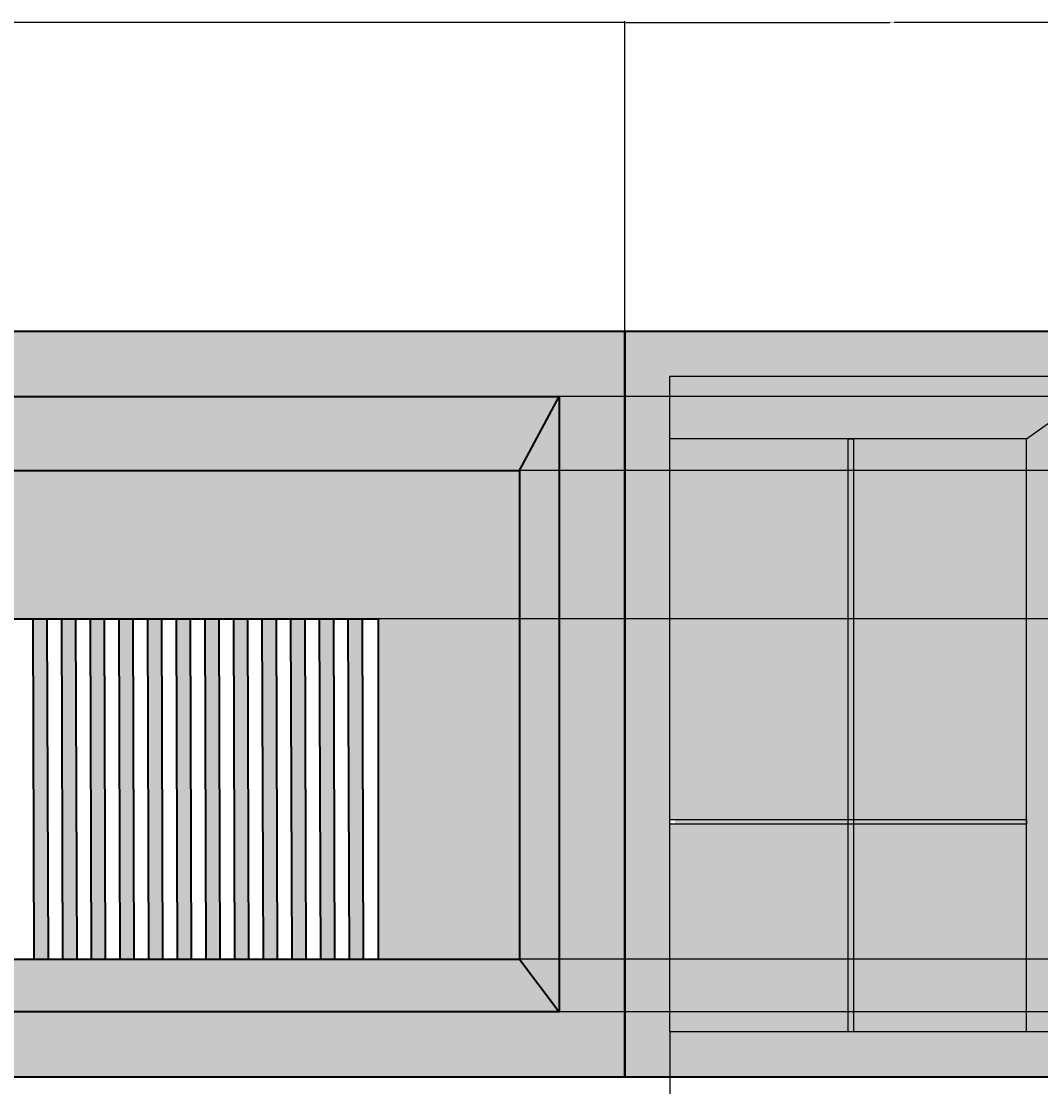
# Model space of a CAD drawing. Units: feet. Extents: x 1141 to 2858, y 751 to 1654.
# Tile 7 of 13: x 1916 to 2096, y 1466 to 1654. Entities that reach past the tile are written whole.
import ezdxf

# ---------------------------------------------------------------- set-up
doc = ezdxf.new("R2010")
doc.units = ezdxf.units.FT
for name, color, linetype, lineweight in [('A-ANNO-DIMS', 2, 'Continuous', 18), ('A-ELEV', 7, 'Continuous', 35), ('A-ELEV-PATT', 8, 'Continuous', 13), ('A-GLAZ', 4, 'Continuous', 25)]:
    doc.layers.add(name, color=color, linetype=linetype, lineweight=lineweight)
doc.styles.get("Standard").update_dxf_attribs({"font": 'arial.ttf'})
doc.dimstyles.get("Standard").update_dxf_attribs({"dimtxt": 0.18, "dimasz": 0.18, "dimexe": 0.18, "dimexo": 0.0625, "dimgap": 0.09, "dimtad": 0, "dimtih": 1, "dimtoh": 1, "dimdec": 1, "dimzin": 0, "dimdsep": 46, "dimlunit": 3, "dimtxsty": 'Standard', "dimcen": 0.09, "dimadec": 0, "dimazin": 0, "dimtfac": 1, "dimtdec": 1, "dimtofl": 0, "dimtmove": 0, "dimatfit": 3, "dimfxl": 1, "dimtolj": 1, "dimtzin": 0, "dimarcsym": 0})

# ---------------------------------------------------------------- blocks, each defined once
blk = doc.blocks.new('WIN-SIDE-A')
blk.add_line((63.09, 104.94), (78.57, 116.03))
blk.add_line((63.09, 104.94), (78.57, 116.03))
for points in [[(78.57, 0), (0, 0), (0, 116.03), (78.57, 116.03)], [(78.57, 0), (0, 0), (0, 116.03), (78.57, 116.03)], [(31.54, 104.94), (32.46, 104.94), (32.46, 0), (31.54, 0)], [(0, 37.61), (63.09, 37.61), (63.09, 36.79), (0, 36.79)]]:
    blk.add_lwpolyline(points, close=True)
for points in [[(63.09, 0), (63.09, 104.94), (0, 104.94)], [(63.09, 0), (63.09, 104.94), (0, 104.94)], [(31.54, 37.61), (31.54, 104.94), (32.46, 104.94), (32.46, 37.61)], [(31.54, 36.79), (0, 36.79), (0, 37.61), (31.54, 37.61)], [(32.46, 36.79), (32.46, 0), (31.54, 0), (31.54, 36.79)], [(32.46, 37.61), (63.09, 37.61), (63.09, 36.79), (32.46, 36.79)]]:
    blk.add_lwpolyline(points)
blk = doc.blocks.new('*D15')
at = {"layer": 'A-ANNO-DIMS', "color": 0, "lineweight": -2, "transparency": 16777216}
for p, q in [((2030.85, 1475.38), (2030.85, 1457.85)), ((2109.42, 1475.38), (2109.42, 1457.85)), ((2031.03, 1458.03), (2069.61, 1458.03)), ((2109.24, 1458.03), (2070.66, 1458.03))]:
    blk.add_line(p, q, dxfattribs=at)
at = {"layer": 'A-ANNO-DIMS', "color": 0, "transparency": 16777216}
for points in [[(2031.03, 1458.06), (2031.03, 1458), (2030.85, 1458.03)], [(2109.24, 1458.06), (2109.24, 1458), (2109.42, 1458.03)]]:
    blk.add_solid(points, dxfattribs=at)
at = {"layer": 'Defpoints', "color": 0, "transparency": 16777216}
for p in [(2030.85, 1475.44), (2109.42, 1475.44), (2109.42, 1458.03)]:
    blk.add_point(p, dxfattribs=at)
at = {"layer": 'A-ANNO-DIMS', "color": 0, "transparency": 16777216, "insert": (2070.14, 1458.03), "char_height": 0.18, "attachment_point": 5}
blk.add_mtext('\\A1;79 TYP.', dxfattribs=at)
blk = doc.blocks.new('*D25')
at = {"layer": 'A-ANNO-DIMS', "color": 0, "lineweight": -2, "transparency": 16777216}
for p, q in [((1726.03, 1599.52), (1726.03, 1654.28)), ((1726.21, 1654.1), (1873.98, 1654.1)), ((2022.69, 1654.1), (1874.91, 1654.1)), ((2022.87, 1599.52), (2022.87, 1654.28))]:
    blk.add_line(p, q, dxfattribs=at)
at = {"layer": 'A-ANNO-DIMS', "color": 0, "transparency": 16777216}
for points in [[(1726.21, 1654.13), (1726.21, 1654.07), (1726.03, 1654.1)], [(2022.69, 1654.13), (2022.69, 1654.07), (2022.87, 1654.1)]]:
    blk.add_solid(points, dxfattribs=at)
at = {"layer": 'Defpoints', "color": 0, "transparency": 16777216}
for p in [(2022.87, 1654.1), (1726.03, 1599.45), (2022.87, 1599.45)]:
    blk.add_point(p, dxfattribs=at)
at = {"layer": 'A-ANNO-DIMS', "color": 0, "transparency": 16777216, "insert": (1874.45, 1654.1), "char_height": 0.18, "attachment_point": 5}
blk.add_mtext('\\A1;296.83', dxfattribs=at)
blk = doc.blocks.new('*D26')
at = {"layer": 'A-ANNO-DIMS', "color": 0, "lineweight": -2, "transparency": 16777216}
for p, q in [((2022.87, 1599.52), (2022.87, 1654.28)), ((2023.05, 1654.1), (2069.74, 1654.1)), ((2117.23, 1654.1), (2070.53, 1654.1)), ((2117.41, 1599.52), (2117.41, 1654.28))]:
    blk.add_line(p, q, dxfattribs=at)
at = {"layer": 'A-ANNO-DIMS', "color": 0, "transparency": 16777216}
for points in [[(2023.05, 1654.13), (2023.05, 1654.07), (2022.87, 1654.1)], [(2117.23, 1654.13), (2117.23, 1654.07), (2117.41, 1654.1)]]:
    blk.add_solid(points, dxfattribs=at)
at = {"layer": 'Defpoints', "color": 0, "transparency": 16777216}
for p in [(2117.41, 1654.1), (2022.87, 1599.45), (2117.41, 1599.45)]:
    blk.add_point(p, dxfattribs=at)
at = {"layer": 'A-ANNO-DIMS', "color": 0, "transparency": 16777216, "insert": (2070.14, 1654.1), "char_height": 0.18, "attachment_point": 5}
blk.add_mtext('\\A1;94.54', dxfattribs=at)
blk = doc.blocks.new('*D39')
at = {"layer": 'A-ANNO-DIMS', "color": 0, "lineweight": -2, "transparency": 16777216}
for p, q in [((2319.24, 1599.45), (1668.14, 1599.45)), ((1668.32, 1599.27), (1668.32, 1202.86)), ((1668.32, 806.08), (1668.32, 1202.49)), ((2319.24, 805.9), (1668.14, 805.9))]:
    blk.add_line(p, q, dxfattribs=at)
at = {"layer": 'A-ANNO-DIMS', "color": 0, "transparency": 16777216}
for points in [[(1668.29, 1599.27), (1668.35, 1599.27), (1668.32, 1599.45)], [(1668.29, 806.08), (1668.35, 806.08), (1668.32, 805.9)]]:
    blk.add_solid(points, dxfattribs=at)
at = {"layer": 'Defpoints', "color": 0, "transparency": 16777216}
for p in [(1668.32, 1599.45), (2319.3, 1599.45), (2319.3, 805.9)]:
    blk.add_point(p, dxfattribs=at)
at = {"layer": 'A-ANNO-DIMS', "color": 0, "transparency": 16777216, "insert": (1668.32, 1202.68), "char_height": 0.18, "attachment_point": 5}
blk.add_mtext('\\A1;793.6', dxfattribs=at)
blk = doc.blocks.new('*D48')
at = {"layer": 'A-ANNO-DIMS', "color": 0, "lineweight": -2, "transparency": 16777216}
for p, q in [((2330.82, 1479.03), (1668.14, 1479.03)), ((1668.32, 1478.85), (1668.32, 1473.42)), ((1668.32, 1467.63), (1668.32, 1473.06)), ((2319.24, 1467.45), (1668.14, 1467.45))]:
    blk.add_line(p, q, dxfattribs=at)
at = {"layer": 'A-ANNO-DIMS', "color": 0, "transparency": 16777216}
for points in [[(1668.29, 1478.85), (1668.35, 1478.85), (1668.32, 1479.03)], [(1668.29, 1467.63), (1668.35, 1467.63), (1668.32, 1467.45)]]:
    blk.add_solid(points, dxfattribs=at)
at = {"layer": 'Defpoints', "color": 0, "transparency": 16777216}
for p in [(1668.32, 1479.03), (2330.88, 1479.03), (2319.3, 1467.45)]:
    blk.add_point(p, dxfattribs=at)
at = {"layer": 'A-ANNO-DIMS', "color": 0, "transparency": 16777216, "insert": (1668.32, 1473.24), "char_height": 0.18, "attachment_point": 5}
blk.add_mtext('\\A1;11.58', dxfattribs=at)
blk = doc.blocks.new('*D49')
at = {"layer": 'A-ANNO-DIMS', "color": 0, "lineweight": -2, "transparency": 16777216}
for p, q in [((2347.45, 1488.33), (1668.14, 1488.33)), ((1668.32, 1488.15), (1668.32, 1483.86)), ((1668.32, 1479.21), (1668.32, 1483.5)), ((2330.82, 1479.03), (1668.14, 1479.03))]:
    blk.add_line(p, q, dxfattribs=at)
at = {"layer": 'A-ANNO-DIMS', "color": 0, "transparency": 16777216}
for points in [[(1668.29, 1488.15), (1668.35, 1488.15), (1668.32, 1488.33)], [(1668.29, 1479.21), (1668.35, 1479.21), (1668.32, 1479.03)]]:
    blk.add_solid(points, dxfattribs=at)
at = {"layer": 'Defpoints', "color": 0, "transparency": 16777216}
for p in [(1668.32, 1488.33), (2347.51, 1488.33), (2330.88, 1479.03)]:
    blk.add_point(p, dxfattribs=at)
at = {"layer": 'A-ANNO-DIMS', "color": 0, "transparency": 16777216, "insert": (1668.32, 1483.68), "char_height": 0.18, "attachment_point": 5}
blk.add_mtext('\\A1;9.293', dxfattribs=at)
blk = doc.blocks.new('*D50')
at = {"layer": 'A-ANNO-DIMS', "color": 0, "lineweight": -2, "transparency": 16777216}
for p, q in [((2356.58, 1548.54), (1668.14, 1548.54)), ((1668.32, 1548.36), (1668.32, 1518.62)), ((1668.32, 1488.51), (1668.32, 1518.25)), ((2347.45, 1488.33), (1668.14, 1488.33))]:
    blk.add_line(p, q, dxfattribs=at)
at = {"layer": 'A-ANNO-DIMS', "color": 0, "transparency": 16777216}
for points in [[(1668.29, 1548.36), (1668.35, 1548.36), (1668.32, 1548.54)], [(1668.29, 1488.51), (1668.35, 1488.51), (1668.32, 1488.33)]]:
    blk.add_solid(points, dxfattribs=at)
at = {"layer": 'Defpoints', "color": 0, "transparency": 16777216}
for p in [(1668.32, 1548.54), (2356.64, 1548.54), (2347.51, 1488.33)]:
    blk.add_point(p, dxfattribs=at)
at = {"layer": 'A-ANNO-DIMS', "color": 0, "transparency": 16777216, "insert": (1668.32, 1518.43), "char_height": 0.18, "attachment_point": 5}
blk.add_mtext('\\A1;60.22', dxfattribs=at)
blk = doc.blocks.new('*D51')
at = {"layer": 'A-ANNO-DIMS', "color": 0, "lineweight": -2, "transparency": 16777216}
for p, q in [((2347.45, 1574.77), (1668.14, 1574.77)), ((1668.32, 1574.59), (1668.32, 1561.84)), ((1668.32, 1548.72), (1668.32, 1561.47)), ((2356.58, 1548.54), (1668.14, 1548.54))]:
    blk.add_line(p, q, dxfattribs=at)
at = {"layer": 'A-ANNO-DIMS', "color": 0, "transparency": 16777216}
for points in [[(1668.29, 1574.59), (1668.35, 1574.59), (1668.32, 1574.77)], [(1668.29, 1548.72), (1668.35, 1548.72), (1668.32, 1548.54)]]:
    blk.add_solid(points, dxfattribs=at)
at = {"layer": 'Defpoints', "color": 0, "transparency": 16777216}
for p in [(1668.32, 1574.77), (2347.51, 1574.77), (2356.64, 1548.54)]:
    blk.add_point(p, dxfattribs=at)
at = {"layer": 'A-ANNO-DIMS', "color": 0, "transparency": 16777216, "insert": (1668.32, 1561.66), "char_height": 0.18, "attachment_point": 5}
blk.add_mtext('\\A1;26.23', dxfattribs=at)
blk = doc.blocks.new('*D52')
at = {"layer": 'A-ANNO-DIMS', "color": 0, "lineweight": -2, "transparency": 16777216}
for p, q in [((2330.82, 1587.87), (1668.14, 1587.87)), ((1668.32, 1587.69), (1668.32, 1581.5)), ((1668.32, 1574.95), (1668.32, 1581.14)), ((2347.45, 1574.77), (1668.14, 1574.77))]:
    blk.add_line(p, q, dxfattribs=at)
at = {"layer": 'A-ANNO-DIMS', "color": 0, "transparency": 16777216}
for points in [[(1668.29, 1587.69), (1668.35, 1587.69), (1668.32, 1587.87)], [(1668.29, 1574.95), (1668.35, 1574.95), (1668.32, 1574.77)]]:
    blk.add_solid(points, dxfattribs=at)
at = {"layer": 'Defpoints', "color": 0, "transparency": 16777216}
for p in [(1668.32, 1587.87), (2330.88, 1587.87), (2347.51, 1574.77)]:
    blk.add_point(p, dxfattribs=at)
at = {"layer": 'A-ANNO-DIMS', "color": 0, "transparency": 16777216, "insert": (1668.32, 1581.32), "char_height": 0.18, "attachment_point": 5}
blk.add_mtext('\\A1;13.102', dxfattribs=at)
blk = doc.blocks.new('*D53')
at = {"layer": 'A-ANNO-DIMS', "color": 0, "lineweight": -2, "transparency": 16777216}
for p, q in [((2319.24, 1599.45), (1668.14, 1599.45)), ((1668.32, 1599.27), (1668.32, 1593.84)), ((1668.32, 1588.05), (1668.32, 1593.48)), ((2330.82, 1587.87), (1668.14, 1587.87))]:
    blk.add_line(p, q, dxfattribs=at)
at = {"layer": 'A-ANNO-DIMS', "color": 0, "transparency": 16777216}
for points in [[(1668.29, 1599.27), (1668.35, 1599.27), (1668.32, 1599.45)], [(1668.29, 1588.05), (1668.35, 1588.05), (1668.32, 1587.87)]]:
    blk.add_solid(points, dxfattribs=at)
at = {"layer": 'Defpoints', "color": 0, "transparency": 16777216}
for p in [(1668.32, 1599.45), (2319.3, 1599.45), (2330.88, 1587.87)]:
    blk.add_point(p, dxfattribs=at)
at = {"layer": 'A-ANNO-DIMS', "color": 0, "transparency": 16777216, "insert": (1668.32, 1593.66), "char_height": 0.18, "attachment_point": 5}
blk.add_mtext('\\A1;11.58', dxfattribs=at)

msp = doc.modelspace()

# ---------------------------------------------------------------- hatches: boundary and pattern name
at = {"layer": 'A-ELEV-PATT'}
h = msp.add_hatch(color=256, dxfattribs=at)
h.dxf.hatch_style = 1
h.paths.add_polyline_path([(2206.032, 1599.4527), (2192.689, 1599.4527), (2192.689, 919.339), (2206.032, 919.339)])
h.paths.add_polyline_path([(2190.2416, 1599.4527), (2175.463, 1599.4527), (2175.463, 919.339), (2190.2416, 919.339)])
h.paths.add_polyline_path([(2173.0156, 1599.4527), (2117.407, 1599.4527), (2117.407, 919.339), (2173.0156, 919.339)])
h.paths.add_polyline_path([(2022.8666, 1057.9008), (1726.032, 1057.9008), (1726.032, 925.9008), (2022.8666, 925.9008)])
h.paths.add_polyline_path([(1737.6123, 937.4811), (1737.6123, 1046.3205), (2011.2863, 1046.3205), (2011.2863, 937.4811)], flags=16)
h.paths.add_polyline_path([(1754.2423, 946.7736), (1754.2423, 1033.2183), (2004.2323, 1033.2183), (2004.2323, 946.7736), (2004.3069, 946.6754), (1906.0824, 946.6754)], flags=0)
h.paths.add_polyline_path([(1900.5421, 946.7736), (1857.5566, 946.7736), (1857.5566, 1033.2183), (1900.5421, 1033.2183)], flags=0)
h.paths.add_polyline_path([(1910.8368, 951.4297), (1910.8368, 1022.7957), (1999.478, 1022.7957), (1999.478, 951.4297)], flags=0)
h.paths.add_polyline_path([(1930.8039, 951.4297), (1930.8039, 1022.7957), (1932.373, 1022.7957), (1932.373, 951.4297)], flags=0)
h.paths.add_polyline_path([(1851.6414, 946.7736), (1826.5664, 946.7736), (1826.5664, 967.8234), (1793.4402, 967.8234), (1793.4402, 946.7736), (1790.4043, 946.7736), (1790.4043, 967.8234), (1754.2423, 967.8234), (1754.2423, 970.4796), (1790.4043, 970.4796), (1790.4043, 1033.2183), (1793.4402, 1033.2183), (1793.4402, 970.4796), (1826.5664, 970.4796), (1826.5664, 1033.2183), (1851.6414, 1033.2183)], flags=0)
h.paths.add_polyline_path([(1954.3728, 951.4297), (1954.3728, 1022.7957), (1955.9419, 1022.7957), (1955.9419, 951.4297)], flags=0)
h.paths.add_polyline_path([(1977.7327, 951.4297), (1977.7327, 1022.7957), (1979.3018, 1022.7957), (1979.3018, 951.4297)], flags=0)
h.paths.add_polyline_path([(2022.8666, 1193.2888), (1726.032, 1193.2888), (1726.032, 1061.2888), (2022.8666, 1061.2888)])
h.paths.add_polyline_path([(1737.6123, 1072.869), (1737.6123, 1181.7085), (2011.2863, 1181.7085), (2011.2863, 1072.869)], flags=16)
h.paths.add_polyline_path([(1754.2423, 1082.1616), (1754.2423, 1168.6063), (2004.2323, 1168.6063), (2004.2323, 1082.1616), (2004.3069, 1082.0634), (1906.0824, 1082.0634)], flags=0)
h.paths.add_polyline_path([(1900.5421, 1082.1616), (1857.5566, 1082.1616), (1857.5566, 1168.6063), (1900.5421, 1168.6063)], flags=0)
h.paths.add_polyline_path([(1910.8368, 1086.8177), (1910.8368, 1158.1837), (1999.478, 1158.1837), (1999.478, 1086.8177)], flags=0)
h.paths.add_polyline_path([(1930.8039, 1086.8177), (1930.8039, 1158.1837), (1932.373, 1158.1837), (1932.373, 1086.8177)], flags=0)
h.paths.add_polyline_path([(1851.6414, 1082.1616), (1826.5664, 1082.1616), (1826.5664, 1103.2114), (1793.4402, 1103.2114), (1793.4402, 1082.1616), (1790.4043, 1082.1616), (1790.4043, 1103.2114), (1754.2423, 1103.2114), (1754.2423, 1105.8676), (1790.4043, 1105.8676), (1790.4043, 1168.6063), (1793.4402, 1168.6063), (1793.4402, 1105.8676), (1826.5664, 1105.8676), (1826.5664, 1168.6063), (1851.6414, 1168.6063)], flags=0)
h.paths.add_polyline_path([(1954.3728, 1086.8177), (1954.3728, 1158.1837), (1955.9419, 1158.1837), (1955.9419, 1086.8177)], flags=0)
h.paths.add_polyline_path([(1977.7327, 1086.8177), (1977.7327, 1158.1837), (1979.3018, 1158.1837), (1979.3018, 1086.8177)], flags=0)
h.paths.add_polyline_path([(2022.8666, 1599.4527), (1726.032, 1599.4527), (1726.032, 1467.4527), (2022.8666, 1467.4527)])
h.paths.add_polyline_path([(2011.2863, 1479.033), (1737.6123, 1479.033), (1737.6123, 1587.8725), (2011.2863, 1587.8725)], flags=16)
h.paths.add_polyline_path([(2004.2323, 1488.3255), (1754.2423, 1488.3255), (1754.2423, 1574.7702), (2004.2323, 1574.7702)], flags=0)
h.paths.add_polyline_path([(1829.1345, 1544.6458), (1914.1177, 1544.6458), (1914.1177, 1539.5463), (1830.9097, 1539.5463), (1831.6817, 1537.3286), (1914.1177, 1537.3286), (1914.1177, 1532.2291), (1833.4569, 1532.2291), (1834.229, 1530.0113), (1914.1177, 1530.0113), (1914.1177, 1524.9118), (1836.0042, 1524.9118), (1836.7762, 1522.694), (1914.1177, 1522.694), (1914.1177, 1517.5946), (1838.5514, 1517.5946), (1839.3235, 1515.3768), (1914.1177, 1515.3768), (1914.1177, 1510.2773), (1841.0987, 1510.2773), (1841.8707, 1508.0595), (1914.1177, 1508.0595), (1914.1177, 1502.9601), (1843.6459, 1502.9601), (1844.4179, 1500.7423), (1914.1177, 1500.7423), (1914.1177, 1495.6428), (1846.1931, 1495.6428), (1846.9652, 1493.425), (1914.1177, 1493.425), (1914.1177, 1488.3255), (1848.6593, 1488.3255), (1848.6593, 1488.5583)], flags=0)
h.paths.add_polyline_path([(2117.407, 1464.0647), (1820.5724, 1464.0647), (1820.5724, 1332.0647), (2117.407, 1332.0647)])
h.paths.add_polyline_path([(2105.8267, 1452.4845), (2105.8267, 1343.645), (1832.1527, 1343.645), (1832.1527, 1452.4845)], flags=16)
h.paths.add_polyline_path([(2089.1967, 1439.3822), (2089.1967, 1352.9376), (1937.3566, 1352.9376), (1937.3566, 1352.8393), (1839.1321, 1352.8393), (1839.2067, 1352.9376), (1839.2067, 1439.3822), (1937.3566, 1439.3822)], flags=0)
h.paths.add_polyline_path([(2016.8727, 1439.3822), (2016.8727, 1376.6436), (2049.9988, 1376.6436), (2049.9988, 1439.3822), (2053.0347, 1439.3822), (2053.0347, 1376.6436), (2089.1967, 1376.6436), (2089.1967, 1373.9873), (2053.0347, 1373.9873), (2053.0347, 1352.9376), (2049.9988, 1352.9376), (2049.9988, 1373.9873), (2016.8727, 1373.9873), (2016.8727, 1352.9376), (1991.7976, 1352.9376), (1991.7976, 1439.3822)], flags=0)
h.paths.add_polyline_path([(1985.8824, 1439.3822), (1985.8824, 1352.9376), (1942.8969, 1352.9376), (1942.8969, 1439.3822)], flags=0)
h.paths.add_polyline_path([(1932.6022, 1428.9596), (1932.6022, 1357.5937), (1843.961, 1357.5937), (1843.961, 1428.9596)], flags=0)
h.paths.add_polyline_path([(1912.6351, 1428.9596), (1912.6351, 1357.5937), (1911.066, 1357.5937), (1911.066, 1428.9596)], flags=0)
h.paths.add_polyline_path([(1889.0662, 1428.9596), (1889.0662, 1357.5937), (1887.4971, 1357.5937), (1887.4971, 1428.9596)], flags=0)
h.paths.add_polyline_path([(1865.7063, 1428.9596), (1865.7063, 1357.5937), (1864.1372, 1357.5937), (1864.1372, 1428.9596)], flags=0)
h.paths.add_polyline_path([(2117.407, 1328.6768), (1820.5724, 1328.6768), (1820.5724, 1196.6768), (2117.407, 1196.6768)])
h.paths.add_polyline_path([(2105.8267, 1317.0965), (2105.8267, 1208.257), (1832.1527, 1208.257), (1832.1527, 1317.0965)], flags=16)
h.paths.add_polyline_path([(2089.1967, 1303.9943), (2089.1967, 1217.5496), (1937.3566, 1217.5496), (1937.3566, 1217.4513), (1839.1321, 1217.4513), (1839.2067, 1217.5496), (1839.2067, 1303.9943), (1937.3566, 1303.9943)], flags=0)
h.paths.add_polyline_path([(2016.8727, 1303.9943), (2016.8727, 1241.2556), (2049.9988, 1241.2556), (2049.9988, 1303.9943), (2053.0347, 1303.9943), (2053.0347, 1241.2556), (2089.1967, 1241.2556), (2089.1967, 1238.5993), (2053.0347, 1238.5993), (2053.0347, 1217.5496), (2049.9988, 1217.5496), (2049.9988, 1238.5993), (2016.8727, 1238.5993), (2016.8727, 1217.5496), (1991.7976, 1217.5496), (1991.7976, 1303.9943)], flags=0)
h.paths.add_polyline_path([(1985.8824, 1303.9943), (1985.8824, 1217.5496), (1942.8969, 1217.5496), (1942.8969, 1303.9943)], flags=0)
h.paths.add_polyline_path([(1932.6022, 1293.5716), (1932.6022, 1222.2057), (1843.961, 1222.2057), (1843.961, 1293.5716)], flags=0)
h.paths.add_polyline_path([(1912.6351, 1293.5716), (1912.6351, 1222.2057), (1911.066, 1222.2057), (1911.066, 1293.5716)], flags=0)
h.paths.add_polyline_path([(1889.0662, 1293.5716), (1889.0662, 1222.2057), (1887.4971, 1222.2057), (1887.4971, 1293.5716)], flags=0)
h.paths.add_polyline_path([(1865.7063, 1293.5716), (1865.7063, 1222.2057), (1864.1372, 1222.2057), (1864.1372, 1293.5716)], flags=0)
h.paths.add_polyline_path([(2206.032, 917.3598), (2027.2589, 917.3598), (2027.2589, 805.9008), (2206.032, 805.9008)])
h.paths.add_polyline_path([(1852.1771, 917.3598), (1726.032, 917.3598), (1726.032, 805.9008), (1852.1771, 805.9008)])
h.paths.add_polyline_path([(2063.3101, 1580.3829), (2093.938, 1580.3829), (2093.938, 1513.0494), (2063.3101, 1513.0494)])
h.paths.add_polyline_path([(2063.3101, 1580.3829), (2093.938, 1580.3829), (2093.938, 1513.0494), (2063.3101, 1513.0494)])
h = msp.add_hatch(color=256, dxfattribs=at)
h.dxf.hatch_style = 1
h.paths.add_polyline_path([(2011.2863, 1587.8725), (1737.6123, 1587.8725), (1754.2423, 1574.7702), (2004.2323, 1574.7702)])
h.paths.add_polyline_path([(1754.2423, 1574.7702), (1737.6123, 1587.8725), (1737.6123, 1479.033), (1754.2423, 1488.3255)])
h.paths.add_polyline_path([(2011.2863, 1587.8725), (2004.2323, 1574.7702), (2004.2323, 1488.3255), (2011.2863, 1479.033)])
h.paths.add_polyline_path([(2004.2323, 1488.3255), (1754.2423, 1488.3255), (1737.6123, 1479.033), (2011.2863, 1479.033)])
h.paths.add_polyline_path([(2105.8267, 1452.4845), (1832.1527, 1452.4845), (1839.2067, 1439.3822), (1937.3566, 1439.3822), (2089.1967, 1439.3822)])
h.paths.add_polyline_path([(1839.2067, 1439.3822), (1832.1527, 1452.4845), (1832.1527, 1343.645), (1839.2067, 1352.9376)])
h.paths.add_polyline_path([(2105.8267, 1452.4845), (2089.1967, 1439.3822), (2089.1967, 1352.9376), (2105.8267, 1343.645)])
h.paths.add_polyline_path([(2089.1967, 1352.9376), (1937.3566, 1352.9376), (1937.3566, 1352.8393), (1839.1321, 1352.8393), (1832.1527, 1343.645), (2105.8267, 1343.645)])
h.paths.add_polyline_path([(1942.8969, 1439.3822), (1937.3566, 1439.3822), (1937.3566, 1352.9376), (1942.8969, 1352.9376)])
h.paths.add_polyline_path([(1991.7976, 1439.3822), (1985.8824, 1439.3822), (1985.8824, 1352.9376), (1991.7976, 1352.9376)])
h.paths.add_polyline_path([(2109.4211, 1591.4669), (2030.8524, 1591.4669), (2030.8524, 1580.3829), (2093.938, 1580.3829)])
h.paths.add_polyline_path([(2109.4211, 1591.4669), (2093.938, 1580.3829), (2093.938, 1475.4386), (2109.4211, 1475.4386)])
h.paths.add_polyline_path([(1991.7976, 1303.9943), (1985.8824, 1303.9943), (1985.8824, 1217.5496), (1991.7976, 1217.5496)])
h.paths.add_polyline_path([(1942.8969, 1303.9943), (1937.3566, 1303.9943), (1937.3566, 1217.5496), (1942.8969, 1217.5496)])
h.paths.add_polyline_path([(2105.8267, 1317.0965), (1832.1527, 1317.0965), (1839.2067, 1303.9943), (1937.3566, 1303.9943), (2089.1967, 1303.9943)])
h.paths.add_polyline_path([(1839.2067, 1303.9943), (1832.1527, 1317.0965), (1832.1527, 1208.257), (1839.2067, 1217.5496)])
h.paths.add_polyline_path([(2089.1967, 1217.5496), (1937.3566, 1217.5496), (1937.3566, 1217.4513), (1839.1321, 1217.4513), (1832.1527, 1208.257), (2105.8267, 1208.257)])
h.paths.add_polyline_path([(2105.8267, 1317.0965), (2089.1967, 1303.9943), (2089.1967, 1217.5496), (2105.8267, 1208.257)])
h.paths.add_polyline_path([(1754.2423, 1168.6063), (1737.6123, 1181.7085), (1737.6123, 1072.869), (1754.2423, 1082.1616)])
h.paths.add_polyline_path([(2011.2863, 1181.7085), (1737.6123, 1181.7085), (1754.2423, 1168.6063), (2004.2323, 1168.6063)])
h.paths.add_polyline_path([(2011.2863, 1181.7085), (2004.2323, 1168.6063), (2004.2323, 1082.1616), (2011.2863, 1072.869)])
h.paths.add_polyline_path([(2004.3069, 1082.0634), (1906.0824, 1082.0634), (1754.2423, 1082.1616), (1737.6123, 1072.869), (2011.2863, 1072.869)])
h.paths.add_polyline_path([(1906.0824, 1168.6063), (1900.5421, 1168.6063), (1900.5421, 1082.1616), (1906.0824, 1082.1616)])
h.paths.add_polyline_path([(1857.5566, 1168.6063), (1851.6414, 1168.6063), (1851.6414, 1082.1616), (1857.5566, 1082.1616)])
h.paths.add_polyline_path([(1906.0824, 1033.2183), (1900.5421, 1033.2183), (1900.5421, 946.7736), (1906.0824, 946.7736)])
h.paths.add_polyline_path([(1857.5566, 1033.2183), (1851.6414, 1033.2183), (1851.6414, 946.7736), (1857.5566, 946.7736)])
h.paths.add_polyline_path([(1754.2423, 1033.2183), (1737.6123, 1046.3205), (1737.6123, 937.4811), (1754.2423, 946.7736)])
h.paths.add_polyline_path([(2011.2863, 1046.3205), (1737.6123, 1046.3205), (1754.2423, 1033.2183), (2004.2323, 1033.2183)])
h.paths.add_polyline_path([(2011.2863, 1046.3205), (2004.2323, 1033.2183), (2004.2323, 946.7736), (2011.2863, 937.4811)])
h.paths.add_polyline_path([(2004.3069, 946.6754), (1906.0824, 946.6754), (1754.2423, 946.7736), (1737.6123, 937.4811), (2011.2863, 937.4811)])
h.paths.add_polyline_path([(2175.463, 1599.4527), (2173.0156, 1599.4527), (2173.0156, 919.339), (2175.463, 919.339)])
h = msp.add_hatch(color=256, dxfattribs=at)
h.dxf.hatch_style = 1
h.paths.add_polyline_path([(2117.407, 1599.4527), (2022.8666, 1599.4527), (2022.8666, 1467.4527), (2117.407, 1467.4527)])
h.paths.add_polyline_path([(2109.4211, 1591.4669), (2109.4211, 1475.4386), (2030.8524, 1475.4386), (2030.8524, 1591.4669)], flags=16)
h.paths.add_polyline_path([(2093.938, 1580.3829), (2093.938, 1512.23), (2063.3101, 1512.23), (2063.3101, 1475.4386), (2062.3952, 1475.4386), (2062.3952, 1512.23), (2030.8524, 1512.23), (2030.8524, 1513.0494), (2062.3952, 1513.0494), (2062.3952, 1580.3829), (2063.3101, 1580.3829)], flags=0)
h = msp.add_hatch(color=256, dxfattribs=at)
h.dxf.hatch_style = 1
h.paths.add_polyline_path([(2062.3952, 1580.3829), (2030.8524, 1580.3829), (2030.8524, 1513.0494), (2062.3952, 1513.0494)])
h.paths.add_polyline_path([(2093.938, 1580.3829), (2063.3101, 1580.3829), (2063.3101, 1513.0494), (2093.938, 1513.0494)])
h.paths.add_polyline_path([(2093.938, 1512.23), (2063.3101, 1512.23), (2063.3101, 1475.4386), (2093.938, 1475.4386)])
h.paths.add_polyline_path([(2062.3952, 1512.23), (2030.8524, 1512.23), (2030.8524, 1475.4386), (2062.3952, 1475.4386)])
h.paths.add_polyline_path([(1780.1289, 1444.9949), (1749.501, 1444.9949), (1749.501, 1377.6615), (1780.1289, 1377.6615)])
h.paths.add_polyline_path([(1812.5866, 1444.9949), (1781.0438, 1444.9949), (1781.0438, 1377.6615), (1812.5866, 1377.6615)])
h.paths.add_polyline_path([(1812.5866, 1376.842), (1781.0438, 1376.842), (1781.0438, 1340.0506), (1812.5866, 1340.0506)])
h.paths.add_polyline_path([(1780.1289, 1376.842), (1749.501, 1376.842), (1749.501, 1340.0506), (1780.1289, 1340.0506)])
h.paths.add_polyline_path([(2105.8267, 1452.4845), (1832.1527, 1452.4845), (1832.1527, 1343.645), (1839.2067, 1352.9376), (1839.2067, 1439.3822), (1937.3566, 1439.3822), (1937.3566, 1352.9376), (1942.8969, 1352.9376), (1942.8969, 1439.3822), (1985.8824, 1439.3822), (1985.8824, 1352.9376), (1991.7976, 1352.9376), (1991.7976, 1439.3822), (2016.8727, 1439.3822), (2016.8727, 1376.6436), (2049.9988, 1376.6436), (2049.9988, 1439.3822), (2053.0347, 1439.3822), (2053.0347, 1376.6436), (2089.1967, 1376.6436), (2089.1967, 1373.9873), (2053.0347, 1373.9873), (2053.0347, 1352.9376), (2049.9988, 1352.9376), (1937.3566, 1352.9376), (1937.3566, 1352.8393), (1839.1321, 1352.8393), (1832.1527, 1343.645), (2105.8267, 1343.645)])
h.paths.add_polyline_path([(2049.9988, 1373.9873), (2016.8727, 1373.9873), (2016.8727, 1352.9376), (2049.9988, 1352.9376)], flags=17)
h.paths.add_polyline_path([(1780.1289, 1309.6069), (1749.501, 1309.6069), (1749.501, 1242.2735), (1780.1289, 1242.2735)])
h.paths.add_polyline_path([(1812.5866, 1309.6069), (1781.0438, 1309.6069), (1781.0438, 1242.2735), (1812.5866, 1242.2735)])
h.paths.add_polyline_path([(1812.5866, 1241.454), (1781.0438, 1241.454), (1781.0438, 1204.6626), (1812.5866, 1204.6626)])
h.paths.add_polyline_path([(1780.1289, 1241.454), (1749.501, 1241.454), (1749.501, 1204.6626), (1780.1289, 1204.6626)])
h.paths.add_polyline_path([(2049.9988, 1303.9943), (2016.8727, 1303.9943), (2016.8727, 1241.2556), (2049.9988, 1241.2556)])
h.paths.add_polyline_path([(2089.1967, 1303.9943), (2053.0347, 1303.9943), (2053.0347, 1241.2556), (2089.1967, 1241.2556)])
h.paths.add_polyline_path([(2089.1967, 1238.5993), (2053.0347, 1238.5993), (2053.0347, 1217.5496), (2089.1967, 1217.5496)])
h.paths.add_polyline_path([(2049.9988, 1238.5993), (2016.8727, 1238.5993), (2016.8727, 1217.5496), (2049.9988, 1217.5496)])
h.paths.add_polyline_path([(2062.3952, 1174.219), (2030.8524, 1174.219), (2030.8524, 1106.8855), (2062.3952, 1106.8855)])
h.paths.add_polyline_path([(2093.938, 1174.219), (2063.3101, 1174.219), (2063.3101, 1106.8855), (2093.938, 1106.8855)])
h.paths.add_polyline_path([(2093.938, 1106.066), (2063.3101, 1106.066), (2063.3101, 1069.2747), (2093.938, 1069.2747)])
h.paths.add_polyline_path([(2062.3952, 1106.066), (2030.8524, 1106.066), (2030.8524, 1069.2747), (2062.3952, 1069.2747)])
h.paths.add_polyline_path([(1906.0824, 1168.6063), (2004.2323, 1168.6063), (2011.2863, 1181.7085), (1737.6123, 1181.7085), (1737.6123, 1072.869), (2011.2863, 1072.869), (2004.3069, 1082.0634), (1906.0824, 1082.0634)])
h.paths.add_polyline_path([(1790.4043, 1168.6063), (1793.4402, 1168.6063), (1793.4402, 1105.8676), (1826.5664, 1105.8676), (1826.5664, 1168.6063), (1851.6414, 1168.6063), (1851.6414, 1082.1616), (1826.5664, 1082.1616), (1826.5664, 1103.2114), (1793.4402, 1103.2114), (1793.4402, 1082.1616), (1790.4043, 1082.1616), (1790.4043, 1103.2114), (1754.2423, 1103.2114), (1754.2423, 1105.8676), (1790.4043, 1105.8676)], flags=16)
h.paths.add_polyline_path([(1857.5566, 1168.6063), (1900.5421, 1168.6063), (1900.5421, 1082.1616), (1857.5566, 1082.1616)], flags=16)
h = msp.add_hatch(color=256, dxfattribs=at)
h.dxf.hatch_style = 1
h.paths.add_polyline_path([(2094.8455, 1513.0294), (2063.3027, 1513.0294), (2063.3027, 1580.3629), (2062.3878, 1580.3629), (2062.3878, 1513.0294), (2031.7599, 1513.0294), (2031.7599, 1512.2099), (2062.3878, 1512.2099), (2062.3878, 1475.4186), (2063.3027, 1475.4186), (2063.3027, 1512.2099), (2094.8455, 1512.2099)])
h = msp.add_hatch(color=256, dxfattribs=at)
h.dxf.hatch_style = 1
h.paths.add_polyline_path([(2004.2323, 1574.7702), (1754.2423, 1574.7702), (1763.3732, 1548.5407), (1979.2491, 1548.5407), (1979.2491, 1488.3255), (2004.2323, 1488.3255)])
h.paths.add_polyline_path([(1754.2423, 1574.7702), (1754.2423, 1488.3255), (1784.3349, 1488.3255)], flags=17)
h.paths.add_polyline_path([(1768.7403, 1548.5407), (1766.0183, 1548.5407), (1786.98, 1488.3255), (1789.702, 1488.3255)], flags=17)
h.paths.add_polyline_path([(1774.1074, 1548.5407), (1771.3854, 1548.5407), (1792.3471, 1488.3255), (1795.0692, 1488.3255)], flags=17)
h.paths.add_polyline_path([(1779.4746, 1548.5407), (1776.7525, 1548.5407), (1797.7142, 1488.3255), (1800.4363, 1488.3255)], flags=17)
h.paths.add_polyline_path([(1784.8417, 1548.5407), (1782.1197, 1548.5407), (1803.0814, 1488.3255), (1805.8034, 1488.3255)], flags=17)
h.paths.add_polyline_path([(1790.2088, 1548.5407), (1787.4868, 1548.5407), (1808.4485, 1488.3255), (1811.1705, 1488.3255)], flags=17)
h.paths.add_polyline_path([(1795.5759, 1548.5407), (1792.8539, 1548.5407), (1813.8156, 1488.3255), (1816.5376, 1488.3255)], flags=17)
h.paths.add_polyline_path([(1800.9431, 1548.5407), (1798.221, 1548.5407), (1819.1827, 1488.3255), (1821.9048, 1488.3255)], flags=17)
h.paths.add_polyline_path([(1806.3102, 1548.5407), (1803.5881, 1548.5407), (1824.5499, 1488.3255), (1827.2719, 1488.3255)], flags=17)
h.paths.add_polyline_path([(1811.6773, 1548.5407), (1808.9553, 1548.5407), (1829.917, 1488.3255), (1832.639, 1488.3255)], flags=17)
h.paths.add_polyline_path([(1817.0444, 1548.5407), (1814.3224, 1548.5407), (1835.2841, 1488.3255), (1838.0061, 1488.3255)], flags=17)
h.paths.add_polyline_path([(1822.4115, 1548.5407), (1819.6895, 1548.5407), (1840.6512, 1488.3255), (1843.3733, 1488.3255)], flags=17)
h.paths.add_polyline_path([(1827.7787, 1548.5407), (1825.0566, 1548.5407), (1846.0183, 1488.3255), (1848.6593, 1488.3255), (1848.6593, 1488.5583)], flags=17)
h.paths.add_polyline_path([(1914.1177, 1544.6458), (1829.1345, 1544.6458), (1830.9097, 1539.5463), (1914.1177, 1539.5463)], flags=17)
h.paths.add_polyline_path([(1914.1177, 1537.3286), (1831.6817, 1537.3286), (1833.4569, 1532.2291), (1914.1177, 1532.2291)], flags=17)
h.paths.add_polyline_path([(1914.1177, 1530.0113), (1834.229, 1530.0113), (1836.0042, 1524.9118), (1914.1177, 1524.9118)], flags=17)
h.paths.add_polyline_path([(1914.1177, 1522.694), (1836.7762, 1522.694), (1838.5514, 1517.5946), (1914.1177, 1517.5946)], flags=17)
h.paths.add_polyline_path([(1914.1177, 1515.3768), (1839.3235, 1515.3768), (1841.0987, 1510.2773), (1914.1177, 1510.2773)], flags=17)
h.paths.add_polyline_path([(1914.1177, 1508.0595), (1841.8707, 1508.0595), (1843.6459, 1502.9601), (1914.1177, 1502.9601)], flags=17)
h.paths.add_polyline_path([(1914.1177, 1500.7423), (1844.4179, 1500.7423), (1846.1931, 1495.6428), (1914.1177, 1495.6428)], flags=17)
h.paths.add_polyline_path([(1914.1177, 1493.425), (1846.9652, 1493.425), (1848.7404, 1488.3255), (1914.1177, 1488.3255)], flags=17)
h.paths.add_polyline_path([(1920.7331, 1548.5407), (1918.1624, 1548.5407), (1918.3509, 1488.3255), (1920.9216, 1488.3255)], flags=17)
h.paths.add_polyline_path([(1925.8019, 1548.5407), (1923.2312, 1548.5407), (1923.4197, 1488.3255), (1925.9904, 1488.3255)], flags=17)
h.paths.add_polyline_path([(1930.8708, 1548.5407), (1928.3, 1548.5407), (1928.4885, 1488.3255), (1931.0592, 1488.3255)], flags=17)
h.paths.add_polyline_path([(1935.9396, 1548.5407), (1933.3688, 1548.5407), (1933.5573, 1488.3255), (1936.128, 1488.3255)], flags=17)
h.paths.add_polyline_path([(1941.0084, 1548.5407), (1938.4376, 1548.5407), (1938.6261, 1488.3255), (1941.1968, 1488.3255)], flags=17)
h.paths.add_polyline_path([(1946.0772, 1548.5407), (1943.5064, 1548.5407), (1943.6949, 1488.3255), (1946.2656, 1488.3255)], flags=17)
h.paths.add_polyline_path([(1951.146, 1548.5407), (1948.5752, 1548.5407), (1948.7637, 1488.3255), (1951.3344, 1488.3255)], flags=17)
h.paths.add_polyline_path([(1956.2148, 1548.5407), (1953.644, 1548.5407), (1953.8325, 1488.3255), (1956.4032, 1488.3255)], flags=17)
h.paths.add_polyline_path([(1961.2836, 1548.5407), (1958.7128, 1548.5407), (1958.9013, 1488.3255), (1961.472, 1488.3255)], flags=17)
h.paths.add_polyline_path([(1966.3524, 1548.5407), (1963.7816, 1548.5407), (1963.9701, 1488.3255), (1966.5408, 1488.3255)], flags=17)
h.paths.add_polyline_path([(1971.4212, 1548.5407), (1968.8504, 1548.5407), (1969.0389, 1488.3255), (1971.6096, 1488.3255)], flags=17)
h.paths.add_polyline_path([(1976.49, 1548.5407), (1973.9192, 1548.5407), (1974.1077, 1488.3255), (1976.6784, 1488.3255)], flags=17)
h.paths.add_polyline_path([(2027.2589, 914.5568), (1852.1771, 914.5568), (1852.1771, 909.9657), (2027.2589, 909.9657)])
h.paths.add_polyline_path([(2027.2589, 906.8659), (1852.1771, 906.8659), (1852.1771, 902.2747), (2027.2589, 902.2747)])
h.paths.add_polyline_path([(2027.2589, 899.1749), (1852.1771, 899.1749), (1852.1771, 894.5837), (2027.2589, 894.5837)])
h.paths.add_polyline_path([(2027.2589, 891.4839), (1852.1771, 891.4839), (1852.1771, 886.8927), (2027.2589, 886.8927)])
h.paths.add_polyline_path([(2027.2589, 883.793), (1852.1771, 883.793), (1852.1771, 879.2018), (2027.2589, 879.2018)])
h.paths.add_polyline_path([(2027.2589, 876.102), (1852.1771, 876.102), (1852.1771, 871.5108), (2027.2589, 871.5108)])
h.paths.add_polyline_path([(2027.2589, 868.411), (1852.1771, 868.411), (1852.1771, 863.8198), (2027.2589, 863.8198)])
h.paths.add_polyline_path([(2027.2589, 860.72), (1852.1771, 860.72), (1852.1771, 856.1289), (2027.2589, 856.1289)])
h.paths.add_polyline_path([(2027.2589, 853.0291), (1852.1771, 853.0291), (1852.1771, 848.4379), (2027.2589, 848.4379)])
h.paths.add_polyline_path([(2027.2589, 845.3381), (1852.1771, 845.3381), (1852.1771, 840.7469), (2027.2589, 840.7469)])
h.paths.add_polyline_path([(2027.2589, 837.6471), (1852.1771, 837.6471), (1852.1771, 833.056), (2027.2589, 833.056)])
h.paths.add_polyline_path([(2027.2589, 829.9562), (1852.1771, 829.9562), (1852.1771, 825.365), (2027.2589, 825.365)])
h.paths.add_polyline_path([(2027.2589, 822.2652), (1852.1771, 822.2652), (1852.1771, 817.674), (2027.2589, 817.674)])
h.paths.add_polyline_path([(2027.2589, 814.5742), (1852.1771, 814.5742), (1852.1771, 809.983), (2027.2589, 809.983)])

# ---------------------------------------------------------------- linework, layer by layer
at = {"layer": 'A-ELEV'}
for p, q in [((2004.2323, 1574.7702), (2011.2863, 1587.8725)), ((2004.2323, 1574.7702), (2011.2863, 1587.8725)), ((1754.2423, 1574.7702), (2004.2323, 1574.7702)), ((1754.2423, 1574.7702), (2004.2323, 1574.7702)), ((2004.2323, 1574.7702), (2004.2323, 1488.2273)), ((2004.2323, 1574.7702), (2004.2323, 1488.2273)), ((1763.3732, 1548.5407), (1979.2491, 1548.5407)), ((1763.3732, 1548.5407), (1979.2491, 1548.5407)), ((1979.2491, 1548.5407), (1979.2491, 1488.3255)), ((1979.2491, 1548.5407), (1979.2491, 1488.3255)), ((1754.2423, 1488.3255), (2004.2323, 1488.3255)), ((1754.2423, 1488.3255), (2004.2323, 1488.3255)), ((2004.2323, 1488.3255), (2011.2863, 1479.033)), ((2004.2323, 1488.3255), (2011.2863, 1479.033))]:
    msp.add_line(p, q, dxfattribs=at)
for points in [[(1726.032, 1599.4527), (2022.8666, 1599.4527), (2022.8666, 1467.4527), (1726.032, 1467.4527)], [(1726.032, 1599.4527), (2022.8666, 1599.4527), (2022.8666, 1467.4527), (1726.032, 1467.4527)], [(2117.407, 1467.4527), (2022.8666, 1467.4527), (2022.8666, 1599.4527), (2117.407, 1599.4527)], [(2117.407, 1467.4527), (2022.8666, 1467.4527), (2022.8666, 1599.4527), (2117.407, 1599.4527)], [(1737.6123, 1587.8725), (2011.2863, 1587.8725), (2011.2863, 1479.033), (1737.6123, 1479.033)], [(1737.6123, 1587.8725), (2011.2863, 1587.8725), (2011.2863, 1479.033), (1737.6123, 1479.033)]]:
    msp.add_lwpolyline(points, close=True, dxfattribs=at)
for points in [[(1918.1624, 1548.5407), (1918.3509, 1488.3255)], [(1918.1624, 1548.5407), (1918.3509, 1488.3255)], [(1920.9216, 1488.3255), (1920.7331, 1548.5407)], [(1920.9216, 1488.3255), (1920.7331, 1548.5407)], [(1923.2312, 1548.5407), (1923.4197, 1488.3255)], [(1923.2312, 1548.5407), (1923.4197, 1488.3255)], [(1925.9904, 1488.3255), (1925.8019, 1548.5407)], [(1925.9904, 1488.3255), (1925.8019, 1548.5407)], [(1928.3, 1548.5407), (1928.4885, 1488.3255)], [(1928.3, 1548.5407), (1928.4885, 1488.3255)], [(1931.0592, 1488.3255), (1930.8708, 1548.5407)], [(1931.0592, 1488.3255), (1930.8708, 1548.5407)], [(1933.3688, 1548.5407), (1933.5573, 1488.3255)], [(1933.3688, 1548.5407), (1933.5573, 1488.3255)], [(1936.128, 1488.3255), (1935.9396, 1548.5407)], [(1936.128, 1488.3255), (1935.9396, 1548.5407)], [(1938.4376, 1548.5407), (1938.6261, 1488.3255)], [(1938.4376, 1548.5407), (1938.6261, 1488.3255)], [(1941.1968, 1488.3255), (1941.0084, 1548.5407)], [(1941.1968, 1488.3255), (1941.0084, 1548.5407)], [(1943.5064, 1548.5407), (1943.6949, 1488.3255)], [(1943.5064, 1548.5407), (1943.6949, 1488.3255)], [(1946.2656, 1488.3255), (1946.0772, 1548.5407)], [(1946.2656, 1488.3255), (1946.0772, 1548.5407)], [(1948.5752, 1548.5407), (1948.7637, 1488.3255)], [(1948.5752, 1548.5407), (1948.7637, 1488.3255)], [(1951.3344, 1488.3255), (1951.146, 1548.5407)], [(1951.3344, 1488.3255), (1951.146, 1548.5407)], [(1953.644, 1548.5407), (1953.8325, 1488.3255)], [(1953.644, 1548.5407), (1953.8325, 1488.3255)], [(1956.4032, 1488.3255), (1956.2148, 1548.5407)], [(1956.4032, 1488.3255), (1956.2148, 1548.5407)], [(1958.7128, 1548.5407), (1958.9013, 1488.3255)], [(1958.7128, 1548.5407), (1958.9013, 1488.3255)], [(1961.472, 1488.3255), (1961.2836, 1548.5407)], [(1961.472, 1488.3255), (1961.2836, 1548.5407)], [(1963.7816, 1548.5407), (1963.9701, 1488.3255)], [(1963.7816, 1548.5407), (1963.9701, 1488.3255)], [(1966.5408, 1488.3255), (1966.3524, 1548.5407)], [(1966.5408, 1488.3255), (1966.3524, 1548.5407)], [(1968.8504, 1548.5407), (1969.0389, 1488.3255)], [(1968.8504, 1548.5407), (1969.0389, 1488.3255)], [(1971.6096, 1488.3255), (1971.4212, 1548.5407)], [(1971.6096, 1488.3255), (1971.4212, 1548.5407)], [(1973.9192, 1548.5407), (1974.1077, 1488.3255)], [(1973.9192, 1548.5407), (1974.1077, 1488.3255)], [(1976.6784, 1488.3255), (1976.49, 1548.5407)], [(1976.6784, 1488.3255), (1976.49, 1548.5407)]]:
    msp.add_lwpolyline(points, dxfattribs=at)

# ---------------------------------------------------------------- block references
at = {"layer": 'A-GLAZ'}
msp.add_blockref('WIN-SIDE-A', (2030.852, 1475.439), dxfattribs=at)

# ---------------------------------------------------------------- dimensions: what is measured, and where the dimension line sits
at = {"layer": 'A-ANNO-DIMS'}
for base, p1, p2, picture, middle in [((2022.8666, 1654.1027), (1726.032, 1599.4527), (2022.8666, 1599.4527), '*D25', (1874.4493, 1654.1027)), ((2117.407, 1654.1027), (2022.8666, 1599.4527), (2117.407, 1599.4527), '*D26', (2070.1368, 1654.1027))]:
    dim = msp.add_linear_dim(base=base, p1=p1, p2=p2, dimstyle='Standard', override={"dimdec": 2, "dimlfac": 1, "dimrnd": 0, "dimzin": 0, "dimdsep": 46, "dimlunit": 2}, dxfattribs=at)
    dim.commit()
    dim.dimension.update_dxf_attribs({"geometry": picture, "text_midpoint": middle})
for base, p1, p2, override, picture, middle in [((1668.3207, 1599.4527), (2319.3013, 805.9008), (2319.3013, 1599.4527), {"dimdec": 1, "dimlfac": 1, "dimrnd": 0, "dimzin": 0, "dimdsep": 46, "dimlunit": 2}, '*D39', (1668.3207, 1202.6768)), ((1668.3207, 1599.4527), (2330.8815, 1587.8725), (2319.3013, 1599.4527), {"dimdec": 2, "dimlfac": 1, "dimrnd": 0, "dimzin": 0, "dimdsep": 46, "dimlunit": 2}, '*D53', (1668.3207, 1593.6626)), ((1668.3207, 1587.8725), (2347.5116, 1574.7702), (2330.8815, 1587.8725), {"dimdec": 3, "dimlfac": 1, "dimrnd": 0, "dimzin": 0, "dimdsep": 46, "dimlunit": 2}, '*D52', (1668.3207, 1581.3214)), ((1668.3207, 1574.7702), (2356.6424, 1548.5407), (2347.5116, 1574.7702), {"dimdec": 2, "dimlfac": 1, "dimrnd": 0, "dimzin": 0, "dimdsep": 46, "dimlunit": 2}, '*D51', (1668.3207, 1561.6555)), ((1668.3207, 1548.5407), (2347.5116, 1488.3255), (2356.6424, 1548.5407), {"dimdec": 2, "dimlfac": 1, "dimrnd": 0, "dimzin": 0, "dimdsep": 46, "dimlunit": 2}, '*D50', (1668.3207, 1518.4331)), ((1668.32065, 1488.32554), (2330.88152, 1479.03299), (2347.51155, 1488.32554), {"dimdec": 3, "dimlfac": 1, "dimrnd": 0, "dimzin": 0, "dimdsep": 46, "dimlunit": 2}, '*D49', (1668.32065, 1483.67926)), ((1668.3207, 1479.033), (2319.3013, 1467.4527), (2330.8815, 1479.033), {"dimdec": 2, "dimlfac": 1, "dimrnd": 0, "dimzin": 0, "dimdsep": 46, "dimlunit": 2}, '*D48', (1668.3207, 1473.2429))]:
    dim = msp.add_linear_dim(base=base, p1=p1, p2=p2, angle=90, dimstyle='Standard', override=override, dxfattribs=at)
    dim.commit()
    dim.dimension.update_dxf_attribs({"geometry": picture, "text_midpoint": middle})
dim = msp.add_linear_dim(base=(2109.4211, 1458.0344), p1=(2030.8524, 1475.4386), p2=(2109.4211, 1475.4386), text='<> TYP.', dimstyle='Standard', override={"dimdec": 0, "dimlfac": 1, "dimrnd": 0, "dimzin": 0, "dimdsep": 46, "dimlunit": 2}, dxfattribs=at)
dim.commit()
dim.dimension.update_dxf_attribs({"geometry": '*D15', "text_midpoint": (2070.1368, 1458.0344)})

doc.saveas('drawing.dxf')
